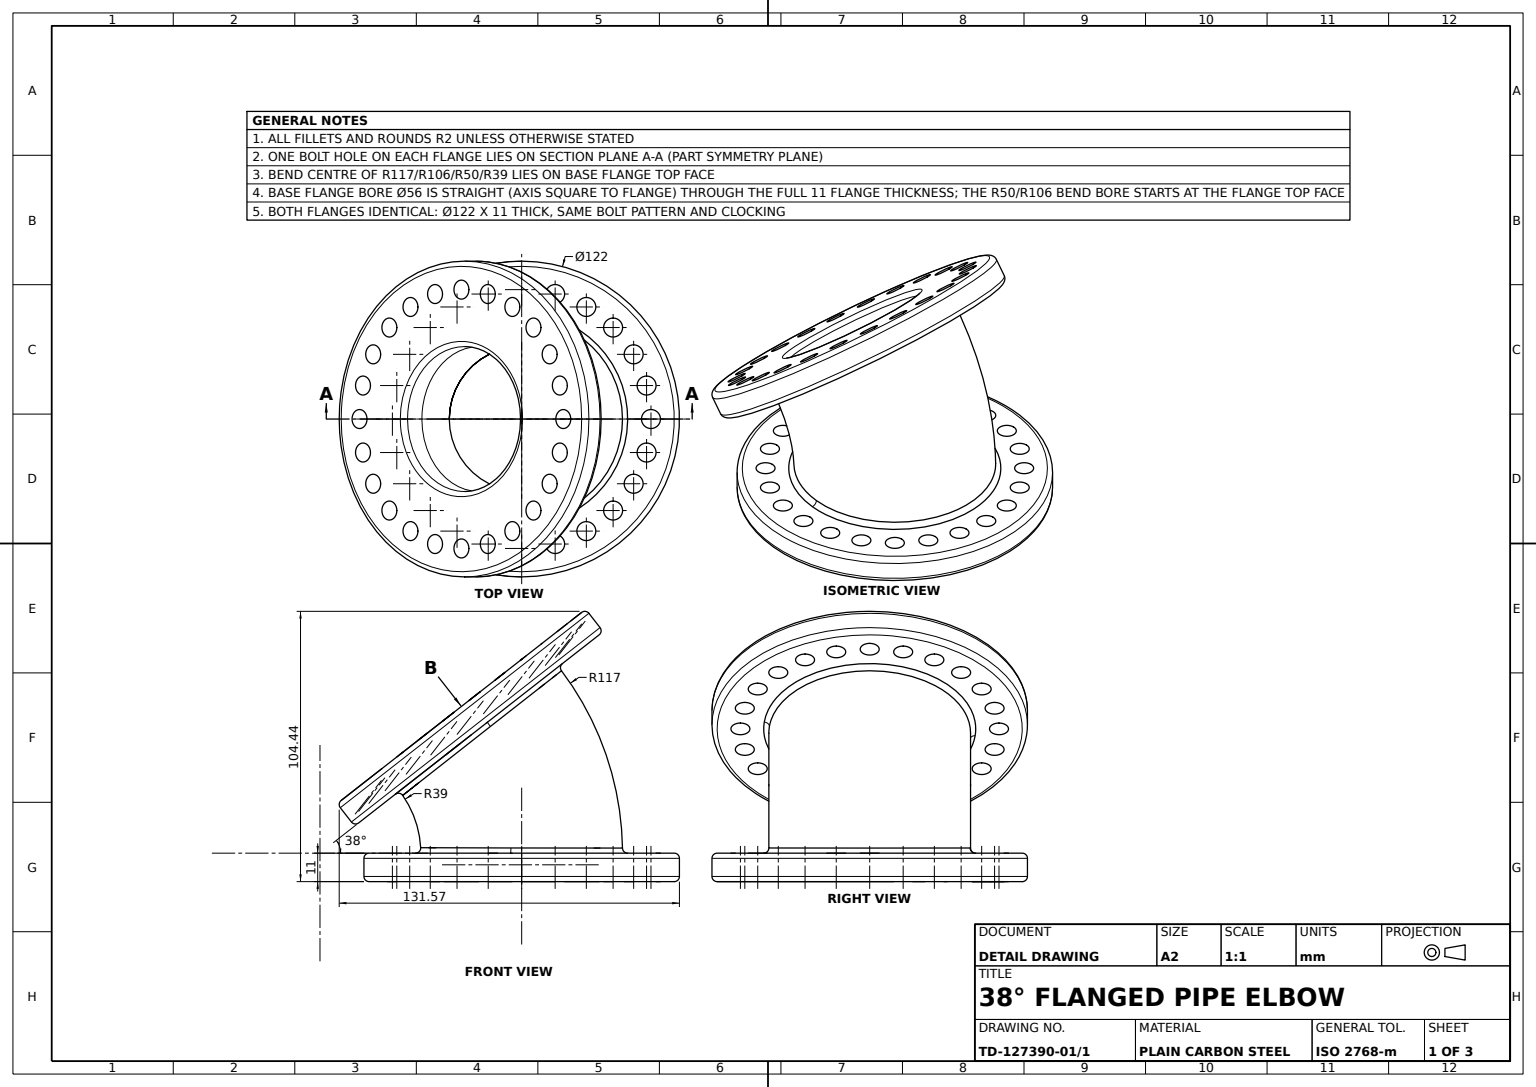
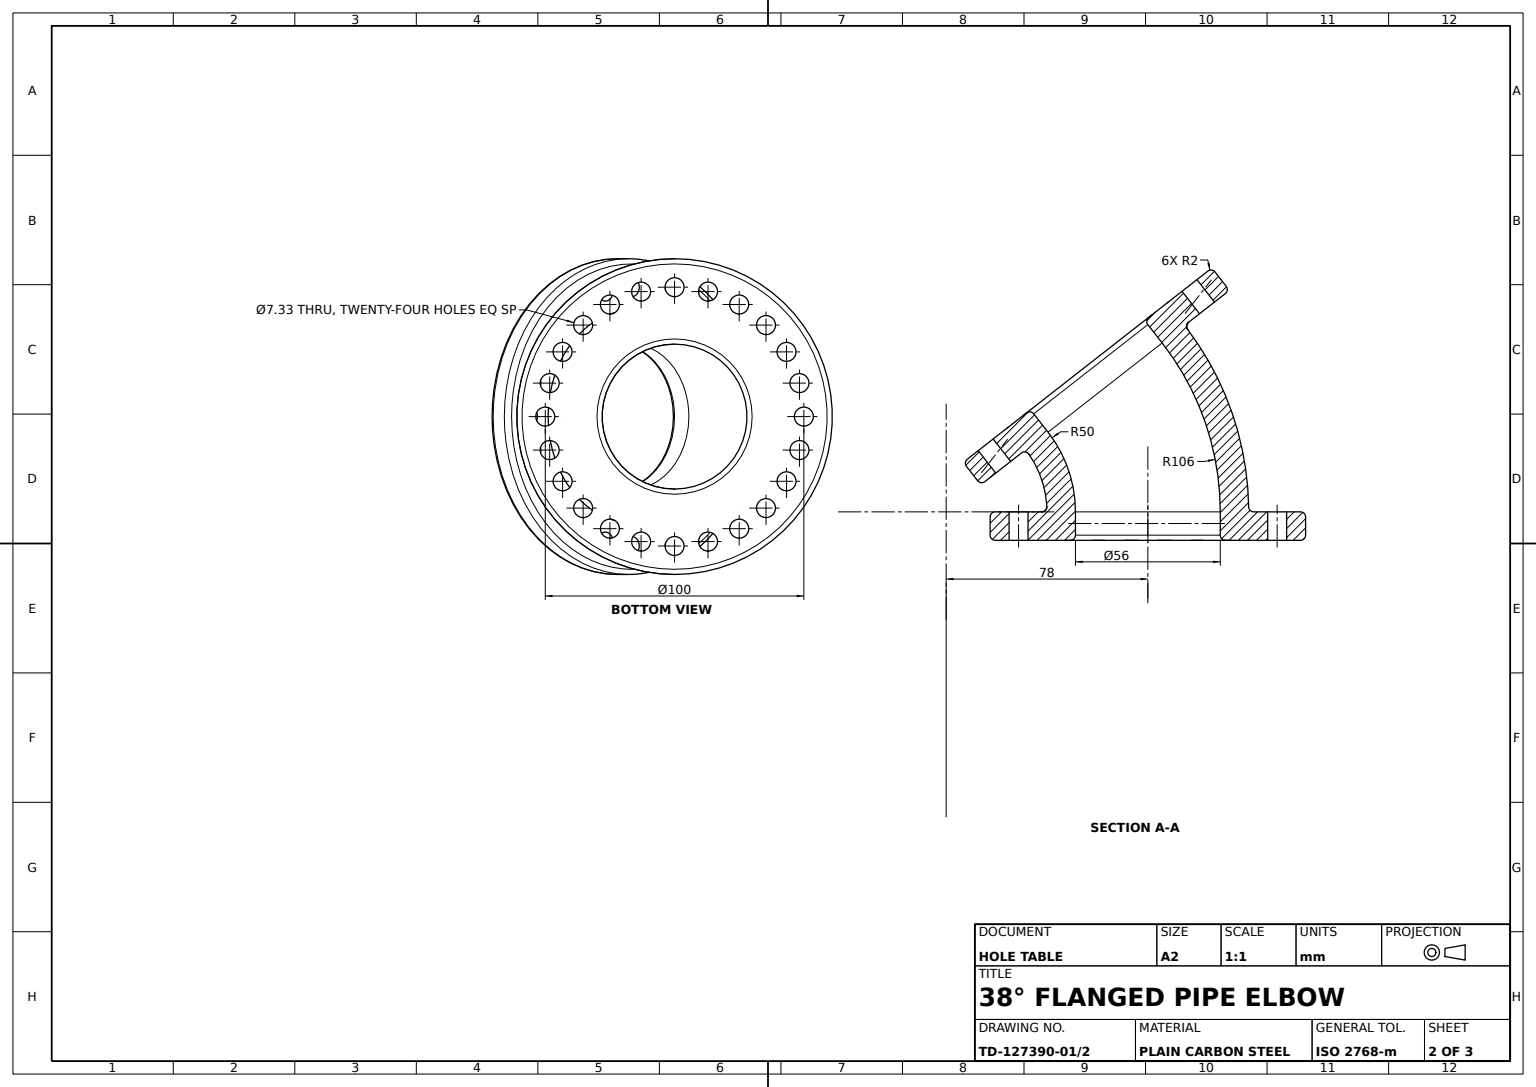
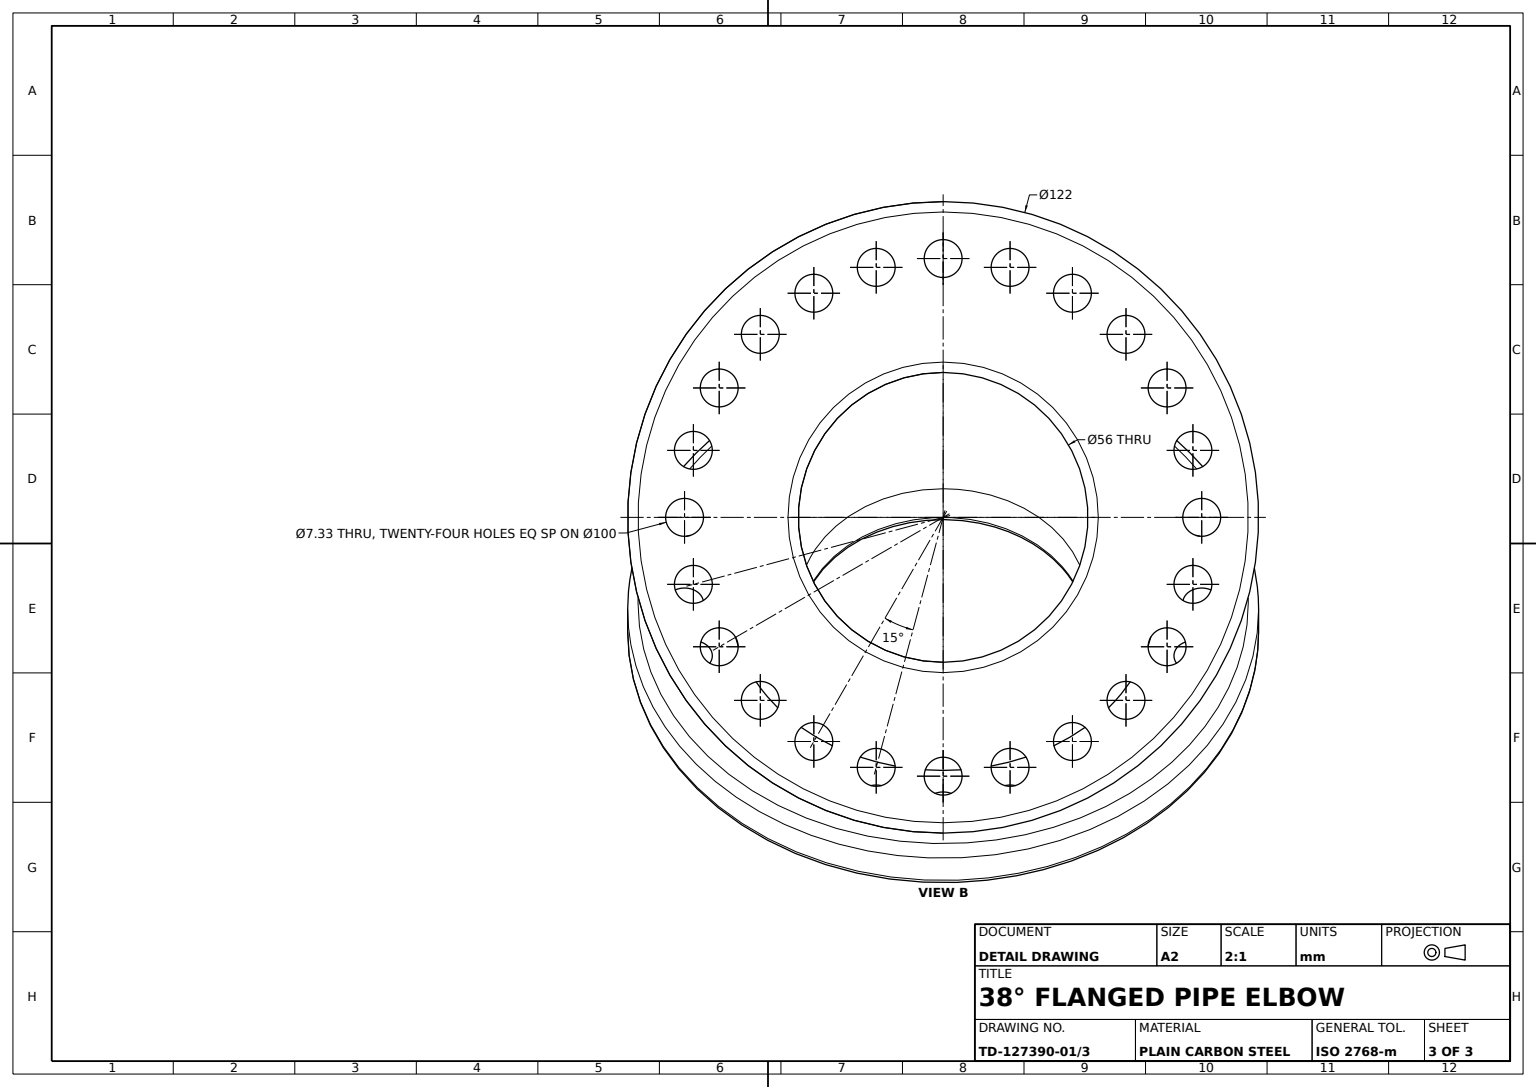
SolidWorks part; units mm, degrees
material "Plain Carbon Steel"
ref_plane "Front Plane" through (0, 0, 0) normal (0, 0, 1) x (1, 0, 0)
ref_plane "Top Plane" through (0, 0, 0) normal (0, 1, 0) x (1, 0, 0)
ref_plane "Right Plane" through (0, 0, 0) normal (1, 0, 0) x (0, 0, -1)
sketch "Base Flange Sketch" plane through (0, 0, 0) normal (0, 1, 0) x (1, 0, 0)
  line L0 (0, 50) -> (0, 0) construction
  circle A0 centre (0, 0) radius 28
  circle A1 centre (0, 0) radius 61
  circle A2 centre (0, 50) radius 3.665
  circle A3 centre (12.941, 48.2963) radius 3.665
  circle A4 centre (25, 43.3013) radius 3.665
  circle A5 centre (35.3553, 35.3553) radius 3.665
  circle A6 centre (43.3013, 25) radius 3.665
  circle A7 centre (48.2963, 12.941) radius 3.665
  circle A8 centre (50, 0) radius 3.665
  circle A9 centre (48.2963, -12.941) radius 3.665
  circle A10 centre (43.3013, -25) radius 3.665
  circle A11 centre (35.3553, -35.3553) radius 3.665
  circle A12 centre (25, -43.3013) radius 3.665
  circle A13 centre (12.941, -48.2963) radius 3.665
  circle A14 centre (0, -50) radius 3.665
  circle A15 centre (-12.941, -48.2963) radius 3.665
  circle A16 centre (-25, -43.3013) radius 3.665
  circle A17 centre (-35.3553, -35.3553) radius 3.665
  circle A18 centre (-43.3013, -25) radius 3.665
  circle A19 centre (-48.2963, -12.941) radius 3.665
  circle A20 centre (-50, 0) radius 3.665
  circle A21 centre (-48.2963, 12.941) radius 3.665
  circle A22 centre (-43.3013, 25) radius 3.665
  circle A23 centre (-35.3553, 35.3553) radius 3.665
  circle A24 centre (-25, 43.3013) radius 3.665
  circle A25 centre (-12.941, 48.2963) radius 3.665
  dimension "D1" = 56
  dimension "D2" = 33
  dimension "D4" = 7.33
  dimension "D3" = 11
  dimension "D5" = 24
extrude "Base Flange 24xØ7.33" add sketch "Base Flange Sketch" against normal blind 11
sketch "Bend Profile Sketch" plane through (0, 0, 0) normal (0, 1, 0) x (1, 0, 0)
  line L0 (-78, 90.6847) -> (-78, -59.4781) construction
  circle A0 centre (0, 0) radius 28 construction
  circle A1 centre (0, 0) radius 28
  circle A2 centre (0, 0) radius 39
  dimension "D2" = 78
  dimension "D1" = 11
revolve "Pipe Bend 38deg" add sketch "Bend Profile Sketch" angle 38 about L0
sketch "End Flange Sketch" plane through (-29.565, 37.8415, 0) normal (-0.6157, 0.788, 0) x (0.788, 0.6157, 0)
  line L0 (16.5352, 50) -> (16.5352, 0) construction
  circle A1 centre (16.5352, 0) radius 28 construction
  circle A2 centre (16.5352, 0) radius 28
  circle A3 centre (16.5352, 0) radius 61
  circle A4 centre (16.5352, 50) radius 3.665
  circle A5 centre (29.4761, 48.2963) radius 3.665
  circle A6 centre (41.5352, 43.3013) radius 3.665
  circle A7 centre (51.8905, 35.3553) radius 3.665
  circle A8 centre (59.8364, 25) radius 3.665
  circle A9 centre (64.8315, 12.941) radius 3.665
  circle A10 centre (66.5352, 0) radius 3.665
  circle A11 centre (64.8315, -12.941) radius 3.665
  circle A12 centre (59.8364, -25) radius 3.665
  circle A13 centre (51.8905, -35.3553) radius 3.665
  circle A14 centre (41.5352, -43.3013) radius 3.665
  circle A15 centre (29.4761, -48.2963) radius 3.665
  circle A16 centre (16.5352, -50) radius 3.665
  circle A17 centre (3.5942, -48.2963) radius 3.665
  circle A18 centre (-8.4648, -43.3013) radius 3.665
  circle A19 centre (-18.8202, -35.3553) radius 3.665
  circle A20 centre (-26.7661, -25) radius 3.665
  circle A21 centre (-31.7611, -12.941) radius 3.665
  circle A22 centre (-33.4648, 0) radius 3.665
  circle A23 centre (-31.7611, 12.941) radius 3.665
  circle A24 centre (-26.7661, 25) radius 3.665
  circle A25 centre (-18.8202, 35.3553) radius 3.665
  circle A26 centre (-8.4648, 43.3013) radius 3.665
  circle A27 centre (3.5942, 48.2963) radius 3.665
  dimension "D1" = 33
  dimension "D2" = 7.33
  dimension "D3" = 11
  dimension "D4" = 24
extrude "End Flange 24xØ7.33" add sketch "End Flange Sketch" along normal blind 11
fillet "Edge Fillets R2" radius 2 8 edges at (0, 0, 61) (0, -11, 61) (0, -11, 28) (-45.3717, 39.4512, 0) (-64.6038, 10.4662, 0) (-71.3761, 19.1344, 0) (-16.5352, 48.0216, 39) (0, 0, 39)
